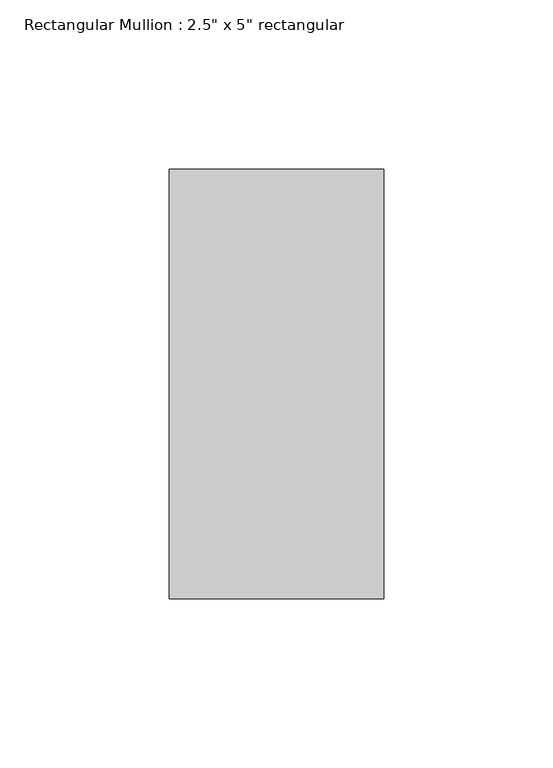
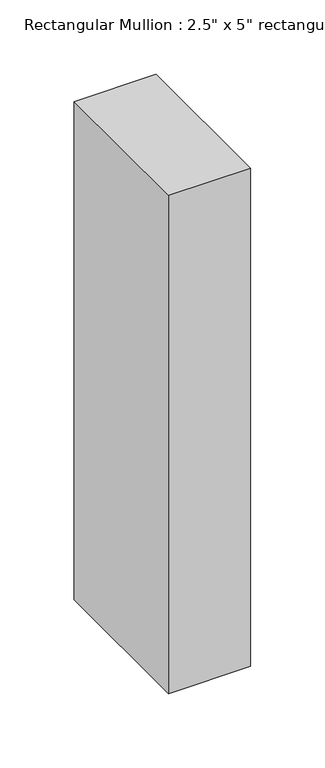
"""IFC4 building model written with IfcOpenShell, lengths in millimetres: member geometry."""

from ifc_helpers import new_model, si_unit, frame, origin, place, context, project, spatial, polyline, outline, extrude, source, transform, mapped, element, save


def member_18dfdc07(model_context):
    return source(origin(), model_context, "Body", "SweptSolid", [
        extrude(outline(polyline([(31.75, 63.5), (31.75, -63.5), (-31.75, -63.5), (-31.75, 63.5), (31.75, 63.5)])), frame((0.0, 0.0, -408.5166667), z_axis=(0.0, 0.0, 1.0), x_axis=(1.0, 0.0, 0.0)), (0.0, 0.0, 1.0), 408.5166667),
    ])


if __name__ == "__main__":
    model = new_model("IFC4")
    model_context = context("Model", 3, world=origin())
    ifc_project = project(units=[si_unit("LENGTHUNIT", "METRE", prefix="MILLI")], contexts=[model_context])
    site = spatial("IfcSite", under=ifc_project)
    building = spatial("IfcBuilding", under=site)
    placement = place(None, origin())
    member_shape = member_18dfdc07(model_context)
    element("IfcMember", 1, ObjectType="Rectangular Mullion : 2.5\" x 5\" rectangular", at=placement, inside=building, context=model_context, shape_type="MappedRepresentation", body=[
        mapped(member_shape, transform((0.0, 0.0, 0.0), x_axis=(1.0, 0.0, 0.0), y_axis=(0.0, 1.0, 0.0), z_axis=(0.0, 0.0, 1.0))),
    ])
    save(model, "model.ifc")

# Revit data of these elements
# Type "Rectangular Mullion : 2.5\" x 5\" rectangular"
#   built-in parameter 1007304 = 0.416667 (stored number, unit not read)
#   built-in parameter 1007301 = 0.104167 (stored number, unit not read)
#   built-in parameter 1007300 = 0.104167 (stored number, unit not read)
# Element 1 (IfcMember, "Rectangular Mullion : 2.5\" x 5\" rectangular")
#   Materials on its faces: "Aluminum"
# Materials
#   "Aluminum": class "Metal", colour RGB 247 247 247, transparency 0, Description = "Aluminum 6061", Cost = 0
